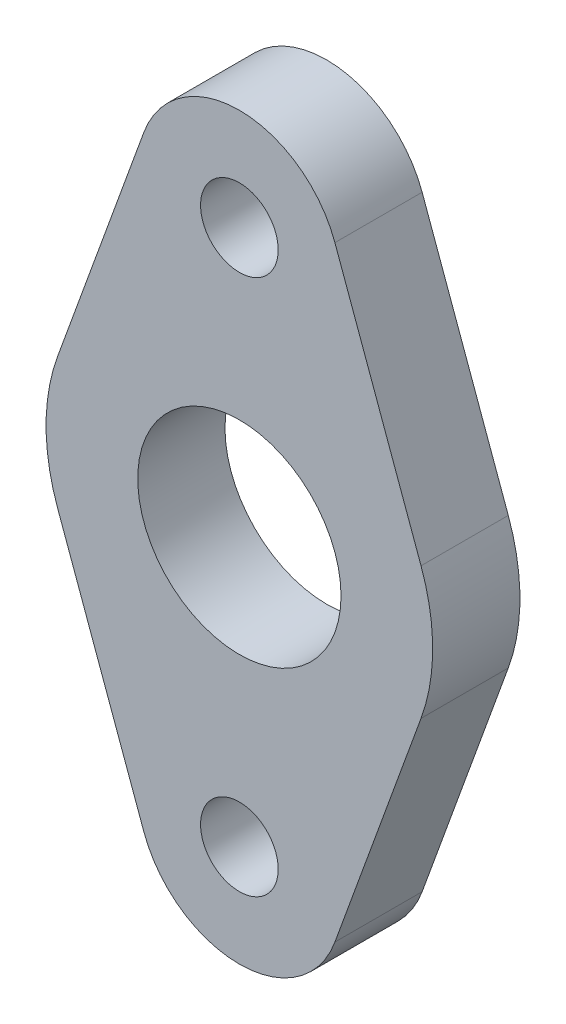
SolidWorks part; units mm, degrees
material "Plain Carbon Steel"
ref_plane "Front Plane" through (0, 0, 0) normal (0, 0, 1) x (1, 0, 0)
ref_plane "Top Plane" through (0, 0, 0) normal (0, 1, 0) x (1, 0, 0)
ref_plane "Right Plane" through (0, 0, 0) normal (1, 0, 0) x (0, 0, -1)
sketch "Flange Outline Sketch" plane through (0, 0, 0) normal (0, 0, 1) x (1, 0, 0)
  line L1 (-11.9352, 37.8407) -> (-22.6956, 8.2543)
  line L2 (11.9352, 37.8407) -> (22.6956, 8.2543)
  line L3 (-11.9352, -37.8407) -> (-22.6956, -8.2543)
  line L4 (11.9352, -37.8407) -> (22.6956, -8.2543)
  arc A0 (-22.6956, 8.2543) -> (-22.6956, -8.2543) centre (0, 0) ccw
  arc A1 (11.9352, 37.8407) -> (-11.9352, 37.8407) centre (0, 33.5) ccw
  arc A2 (11.9352, -37.8407) -> (-11.9352, -37.8407) centre (0, -33.5) cw
  arc A3 (22.6956, -8.2543) -> (22.6956, 8.2543) centre (0, 0) ccw
  dimension "D1" = 48.3
  dimension "D2" = 12.7
  dimension "D5" = 12.7
  dimension "D3" = 33.5
  dimension "D4" = 33.5
  dimension "D6" = 29.5865
  dimension "D7" = 29.5865
  dimension "D8" = 31.4825
  dimension "D9" = 31.4825
extrude "Flange Plate 10.9mm" add sketch "Flange Outline Sketch" along normal blind 10.9
sketch "Bore and Bolt Holes Sketch" plane through (0, 0, 10.9) normal (0, 0, 1) x (1, 0, 0)
  circle A0 centre (0, 33.5) radius 4.85
  circle A1 centre (0, -33.5) radius 4.85
  circle A2 centre (0, 0) radius 12.7
  dimension "D1" = 9.7
  dimension "D2" = 9.7
  dimension "D3" = 25.4
extrude "Bore Ø25.4 and Bolt Holes 2xØ9.7" cut sketch "Bore and Bolt Holes Sketch" against normal blind 49.9
